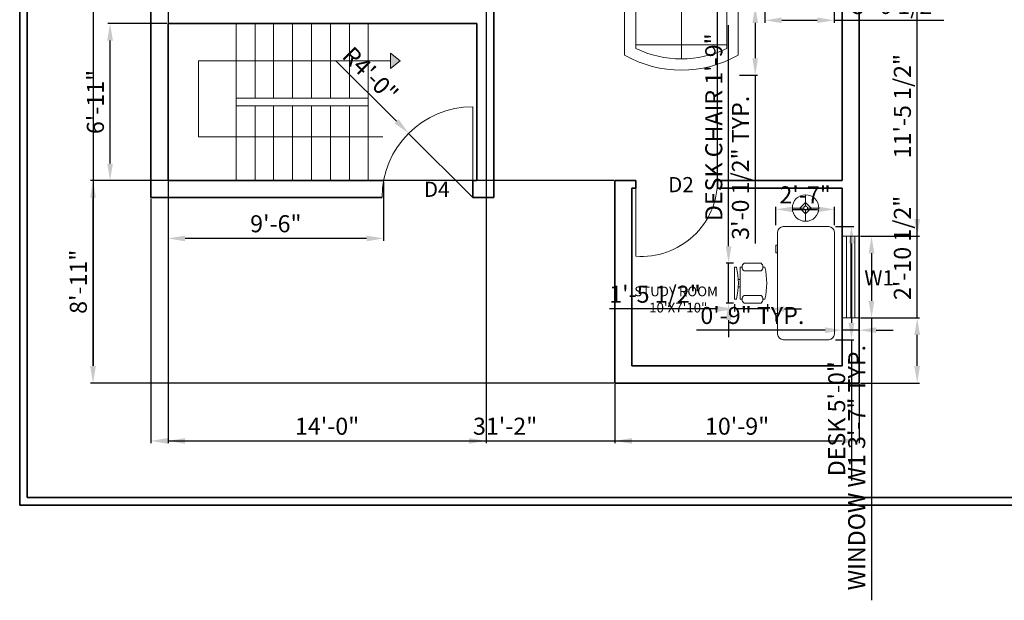
# Model space of a CAD drawing. Units: inches. Extents: x 2396 to 4051, y 1419 to 2191.
# Tile 1 of 7: x 2461 to 2981, y 1419 to 1726. Entities that reach past the tile are written whole.
import ezdxf

# ---------------------------------------------------------------- set-up
doc = ezdxf.new("R2010")
doc.units = ezdxf.units.IN
for name, color, linetype, lineweight in [('A-ANNO-SYMB', 3, 'Continuous', 13), ('A-ANNO-TTLB', 7, 'Continuous', 35), ('A-AREA-IDEN', 6, 'Continuous', 18), ('A-DOOR', 4, 'Continuous', 18), ('A-FLOR-STRS', 7, 'Continuous', 18), ('A-FURN', 8, 'Continuous', 18), ('A-WALL', 7, 'Continuous', 35), ('S-ANNO-DIMS', 2, 'Continuous', 18)]:
    doc.layers.add(name, color=color, linetype=linetype, lineweight=lineweight)
doc.layers.add('A-ANNO-TEXT', color=114, linetype='Continuous', lineweight=18, true_color=0x139b48)
doc.layers.add('A-GLAZ', color=52, linetype='Continuous', lineweight=18, true_color=0xc8c92d)
doc.styles.get("Standard").update_dxf_attribs({"font": 'arial.ttf'})
doc.dimstyles.new('ISO-25', dxfattribs={"dimtxt": 9, "dimasz": 9, "dimexe": 1.25, "dimexo": 0.625, "dimgap": 2, "dimtad": 1, "dimdec": 1, "dimlunit": 4, "dimtxsty": 'Standard', "dimcen": 2.5, "dimadec": 0, "dimazin": 0, "dimtfac": 1, "dimtdec": 1, "dimtmove": 0, "dimatfit": 3, "dimfxl": 1, "dimarcsym": 0})

# ---------------------------------------------------------------- blocks, each defined once
blk = doc.blocks.new('Sofa - Roundback Loveseat 5 ft.')
for p, q in [((0, -32.44198), (0, -5.99998)), ((-24, -33.99998), (-24, -11.46958)), ((-23.9998, -13.38178), (23.99986, -13.38178)), ((24.00004, -33.99998), (24.00004, -11.46958)), ((-24, -32.44198), (24.00004, -32.44198))]:
    blk.add_line(p, q)
for points in [[(-24, -33.99998), (-30, -33.99998), (-30, -7.99998)], [(30.00004, -7.99998), (30.00004, -33.99998), (24.00004, -33.99998)]]:
    blk.add_lwpolyline(points)
for centre, radius, start, end in [((0, -60.24998), 60.24998, 60.13715, 119.8628), ((0, -61.38438), 55.38444, 64.32083, 115.6792)]:
    blk.add_arc(centre, radius, start, end)
blk = doc.blocks.new('Desk - 30 x 60 in.')
for p, q in [((-26.999995, 0), (26.999995, 0)), ((-29.999995, -27), (-29.999995, -3)), ((29.999995, -3), (29.999995, -27)), ((26.999995, -30), (-26.999995, -30)), ((-20.000005, -30), (-20.000005, -31)), ((-20.000005, -31), (-16.000005, -31)), ((-16.000005, -31), (-16.000005, -30)), ((15.999995, -31), (15.999995, -30)), ((19.999995, -31), (15.999995, -31)), ((19.999995, -30), (19.999995, -31))]:
    blk.add_line(p, q)
for centre, start, end in [((-26.499995, -3.5), 98.1301, 171.8699), ((26.499995, -3.5), 8.130102, 81.8699), ((-26.499995, -26.5), 188.1301, 261.8699), ((26.499995, -26.5), 278.1301, 351.8699)]:
    blk.add_arc(centre, 3.535534, start, end)
blk = doc.blocks.new('Lamp - Table')
for p, q in [((0, 7), (0, 1)), ((-1, 0), (-7, 0)), ((0, 3), (-3, 0)), ((-3, 0), (0, -3)), ((3, 0), (0, 3)), ((0, -3), (3, 0)), ((1, 0), (7, 0)), ((0, -1), (0, -7))]:
    blk.add_line(p, q)
for radius in [7, 1]:
    blk.add_circle((0, 0), radius)
blk = doc.blocks.new('Chair - Desk')
for p, q in [((-8.5, 0), (-8.5, -1)), ((-8.5, 0), (8.5, 0)), ((8.5, 0), (8.5, -1)), ((-10.5, -5), (-10.5, -14)), ((-8.5, -3), (-8.5, -4)), ((-8.5, -3), (8.5, -3)), ((-6.5, -14), (-6.5, -5)), ((-2, -3), (-2, -1.9355)), ((2, -1.9576), (2, -3)), ((6.5, -5), (6.5, -14)), ((8.5, -3), (8.5, -4)), ((10.5, -14), (10.5, -5)), ((-8.5, -15), (-8.5, -16)), ((8.5, -15), (8.5, -16))]:
    blk.add_line(p, q)
for centre, radius, start, end in [((-8.5, -6.5), 2.5, 36.8699, 143.1301), ((0, 34.625), 36.625, 256.5803, 283.4197), ((8.5, -6.5), 2.5, 36.8699, 143.1301), ((-8.5, -12.5), 2.5, 216.8699, 323.1301), ((8.5, -12.5), 2.5, 216.8699, 323.1301), ((0, 19.625), 36.625, 256.5803, 283.4197)]:
    blk.add_arc(centre, radius, start, end)
blk = doc.blocks.new('WIN-W1-43P2IN')
for p, q in [((9, 43.2), (0, 43.2)), ((2.25, 0), (2.25, 43.2)), ((4.5, 0), (4.5, 43.2)), ((6.75, 0), (6.75, 43.2)), ((9, 0), (0, 0))]:
    blk.add_line(p, q)
blk = doc.blocks.new('DOOR-D2-40IN')
blk.add_line((0, 40.11), (0, 0.11))
blk.add_arc((3.08, 40.11), 40.12, 265.5948, 0)
blk = doc.blocks.new('*D45')
at = {"layer": 'Defpoints', "color": 0, "transparency": 16777216}
for p in [(2840.06, 1733.59), (2840.06, 1696.93), (2849.06, 1696.93)]:
    blk.add_point(p, dxfattribs=at)
at = {"layer": 'S-ANNO-DIMS', "color": 0, "lineweight": -2, "transparency": 16777216}
for p, q in [((2840.69, 1733.59), (2850.31, 1733.59)), ((2849.06, 1724.59), (2849.06, 1705.93)), ((2840.69, 1696.93), (2850.31, 1696.93)), ((2849.06, 1696.93), (2849.06, 1608.1))]:
    blk.add_line(p, q, dxfattribs=at)
at = {"layer": 'S-ANNO-DIMS', "color": 0, "transparency": 16777216}
for points in [[(2847.56, 1724.59), (2850.56, 1724.59), (2849.06, 1733.59)], [(2847.56, 1705.93), (2850.56, 1705.93), (2849.06, 1696.93)]]:
    blk.add_solid(points, dxfattribs=at)
at = {"layer": 'S-ANNO-DIMS', "color": 0, "transparency": 16777216, "insert": (2842.41, 1648.02), "char_height": 9, "attachment_point": 5, "rotation": 90}
blk.add_mtext('3\'-0 1/2" TYP.', dxfattribs=at)
blk = doc.blocks.new('*D54')
at = {"layer": 'Defpoints', "color": 0, "transparency": 16777216}
for p in [(2903.98, 1611.9), (2903.98, 1568.7), (2910.46, 1568.7)]:
    blk.add_point(p, dxfattribs=at)
at = {"layer": 'S-ANNO-DIMS', "color": 0, "lineweight": -2, "transparency": 16777216}
for p, q in [((2904.61, 1611.9), (2911.71, 1611.9)), ((2910.46, 1602.9), (2910.46, 1577.7)), ((2904.61, 1568.7), (2911.71, 1568.7)), ((2910.46, 1568.7), (2910.46, 1419.46))]:
    blk.add_line(p, q, dxfattribs=at)
at = {"layer": 'S-ANNO-DIMS', "color": 0, "transparency": 16777216}
for points in [[(2908.96, 1602.9), (2911.96, 1602.9), (2910.46, 1611.9)], [(2908.96, 1577.7), (2911.96, 1577.7), (2910.46, 1568.7)]]:
    blk.add_solid(points, dxfattribs=at)
at = {"layer": 'S-ANNO-DIMS', "color": 0, "transparency": 16777216, "insert": (2903.8, 1489.58), "char_height": 9, "attachment_point": 5, "rotation": 90}
blk.add_mtext('WINDOW W1 3\'-7" TYP.', dxfattribs=at)
blk = doc.blocks.new('*D55')
at = {"layer": 'Defpoints', "color": 0, "transparency": 16777216}
for p in [(2894.98, 1568.7), (2903.98, 1568.7), (2894.98, 1562.22)]:
    blk.add_point(p, dxfattribs=at)
at = {"layer": 'S-ANNO-DIMS', "color": 0, "lineweight": -2, "transparency": 16777216}
for p, q in [((2894.98, 1568.08), (2894.98, 1560.97)), ((2903.98, 1568.08), (2903.98, 1560.97)), ((2885.98, 1562.22), (2818.12, 1562.22)), ((2903.98, 1562.22), (2894.98, 1562.22)), ((2912.98, 1562.22), (2921.98, 1562.22))]:
    blk.add_line(p, q, dxfattribs=at)
at = {"layer": 'S-ANNO-DIMS', "color": 0, "transparency": 16777216}
for points in [[(2885.98, 1563.72), (2885.98, 1560.72), (2894.98, 1562.22)], [(2912.98, 1563.72), (2912.98, 1560.72), (2903.98, 1562.22)]]:
    blk.add_solid(points, dxfattribs=at)
at = {"layer": 'S-ANNO-DIMS', "color": 0, "transparency": 16777216, "insert": (2847.55, 1568.82), "char_height": 9, "attachment_point": 5}
blk.add_mtext('0\'-9" TYP.', dxfattribs=at)
blk = doc.blocks.new('*D63')
at = {"layer": 'Defpoints', "color": 0, "transparency": 16777216}
for p in [(2854.1, 1738.57), (2890.77, 1738.57), (2890.77, 1725.97)]:
    blk.add_point(p, dxfattribs=at)
at = {"layer": 'S-ANNO-DIMS', "color": 0, "lineweight": -2, "transparency": 16777216}
for p, q in [((2854.1, 1737.94), (2854.1, 1724.72)), ((2890.77, 1737.94), (2890.77, 1724.72)), ((2863.1, 1725.97), (2881.77, 1725.97)), ((2890.77, 1725.97), (2948.66, 1725.97))]:
    blk.add_line(p, q, dxfattribs=at)
at = {"layer": 'S-ANNO-DIMS', "color": 0, "transparency": 16777216}
for points in [[(2863.1, 1727.47), (2863.1, 1724.47), (2854.1, 1725.97)], [(2881.77, 1727.47), (2881.77, 1724.47), (2890.77, 1725.97)]]:
    blk.add_solid(points, dxfattribs=at)
at = {"layer": 'S-ANNO-DIMS', "color": 0, "transparency": 16777216, "insert": (2924.21, 1732.63), "char_height": 9, "attachment_point": 5}
blk.add_mtext('3\'-0 1/2"', dxfattribs=at)
blk = doc.blocks.new('*D64')
at = {"layer": 'Defpoints', "color": 0, "transparency": 16777216}
for p in [(2890.89, 1617.07), (2890.89, 1557.07), (2899.89, 1557.07)]:
    blk.add_point(p, dxfattribs=at)
at = {"layer": 'S-ANNO-DIMS', "color": 0, "lineweight": -2, "transparency": 16777216}
for p, q in [((2891.51, 1617.07), (2901.14, 1617.07)), ((2899.89, 1608.07), (2899.89, 1566.07)), ((2891.51, 1557.07), (2901.14, 1557.07)), ((2899.89, 1557.07), (2899.89, 1482.86))]:
    blk.add_line(p, q, dxfattribs=at)
at = {"layer": 'S-ANNO-DIMS', "color": 0, "transparency": 16777216}
for points in [[(2898.39, 1608.07), (2901.39, 1608.07), (2899.89, 1617.07)], [(2898.39, 1566.07), (2901.39, 1566.07), (2899.89, 1557.07)]]:
    blk.add_solid(points, dxfattribs=at)
at = {"layer": 'S-ANNO-DIMS', "color": 0, "transparency": 16777216, "insert": (2893.23, 1515.46), "char_height": 9, "attachment_point": 5, "rotation": 90}
blk.add_mtext('DESK 5\'-0"', dxfattribs=at)
blk = doc.blocks.new('*D65')
at = {"layer": 'Defpoints', "color": 0, "transparency": 16777216}
for p in [(2890.89, 1626.07), (2859.89, 1617.07), (2890.89, 1617.07)]:
    blk.add_point(p, dxfattribs=at)
at = {"layer": 'S-ANNO-DIMS', "color": 0, "lineweight": -2, "transparency": 16777216}
for p, q in [((2859.89, 1617.69), (2859.89, 1627.32)), ((2868.89, 1626.07), (2881.89, 1626.07)), ((2890.89, 1617.69), (2890.89, 1627.32))]:
    blk.add_line(p, q, dxfattribs=at)
at = {"layer": 'S-ANNO-DIMS', "color": 0, "transparency": 16777216}
for points in [[(2868.89, 1627.57), (2868.89, 1624.57), (2859.89, 1626.07)], [(2881.89, 1627.57), (2881.89, 1624.57), (2890.89, 1626.07)]]:
    blk.add_solid(points, dxfattribs=at)
at = {"layer": 'S-ANNO-DIMS', "color": 0, "transparency": 16777216, "insert": (2875.39, 1632.58), "char_height": 9, "attachment_point": 5}
blk.add_mtext('2\'-7"', dxfattribs=at)
blk = doc.blocks.new('*D70')
at = {"layer": 'Defpoints', "color": 0, "transparency": 16777216}
for p in [(2834.99, 1597.57), (2838.14, 1597.57), (2838.14, 1576.57)]:
    blk.add_point(p, dxfattribs=at)
at = {"layer": 'S-ANNO-DIMS', "color": 0, "lineweight": -2, "transparency": 16777216}
for p, q in [((2834.99, 1606.57), (2834.99, 1723.39)), ((2837.52, 1597.57), (2833.74, 1597.57)), ((2834.99, 1576.57), (2834.99, 1597.57)), ((2837.52, 1576.57), (2833.74, 1576.57)), ((2834.99, 1567.57), (2834.99, 1558.57))]:
    blk.add_line(p, q, dxfattribs=at)
at = {"layer": 'S-ANNO-DIMS', "color": 0, "transparency": 16777216}
for points in [[(2833.49, 1606.57), (2836.49, 1606.57), (2834.99, 1597.57)], [(2833.49, 1567.57), (2836.49, 1567.57), (2834.99, 1576.57)]]:
    blk.add_solid(points, dxfattribs=at)
at = {"layer": 'S-ANNO-DIMS', "color": 0, "transparency": 16777216, "insert": (2828.34, 1669.48), "char_height": 9, "attachment_point": 5, "rotation": 90}
blk.add_mtext('DESK CHAIR 1\'-9"', dxfattribs=at)
blk = doc.blocks.new('*D71')
at = {"layer": 'Defpoints', "color": 0, "transparency": 16777216}
for p in [(2838.14, 1576.57), (2855.48, 1576.57), (2838.14, 1573.42)]:
    blk.add_point(p, dxfattribs=at)
at = {"layer": 'S-ANNO-DIMS', "color": 0, "lineweight": -2, "transparency": 16777216}
for p, q in [((2838.14, 1575.94), (2838.14, 1572.17)), ((2855.48, 1575.94), (2855.48, 1572.17)), ((2829.14, 1573.42), (2772.09, 1573.42)), ((2855.48, 1573.42), (2838.14, 1573.42)), ((2864.48, 1573.42), (2873.48, 1573.42))]:
    blk.add_line(p, q, dxfattribs=at)
at = {"layer": 'S-ANNO-DIMS', "color": 0, "transparency": 16777216}
for points in [[(2829.14, 1574.92), (2829.14, 1571.92), (2838.14, 1573.42)], [(2864.48, 1574.92), (2864.48, 1571.92), (2855.48, 1573.42)]]:
    blk.add_solid(points, dxfattribs=at)
at = {"layer": 'S-ANNO-DIMS', "color": 0, "transparency": 16777216, "insert": (2796.12, 1580.07), "char_height": 9, "attachment_point": 5}
blk.add_mtext('1\'-5 1/2"', dxfattribs=at)
blk = doc.blocks.new('*D76')
at = {"layer": 'Defpoints', "color": 0, "transparency": 16777216}
for p in [(2529.98, 1632.3), (2903.98, 1534.3), (2903.98, 1503.7)]:
    blk.add_point(p, dxfattribs=at)
at = {"layer": 'S-ANNO-DIMS', "color": 0, "lineweight": -2, "transparency": 16777216}
for p, q in [((2529.98, 1631.68), (2529.98, 1502.45)), ((2903.98, 1533.68), (2903.98, 1502.45)), ((2538.98, 1503.7), (2894.98, 1503.7))]:
    blk.add_line(p, q, dxfattribs=at)
at = {"layer": 'S-ANNO-DIMS', "color": 0, "transparency": 16777216}
for points in [[(2538.98, 1505.2), (2538.98, 1502.2), (2529.98, 1503.7)], [(2894.98, 1505.2), (2894.98, 1502.2), (2903.98, 1503.7)]]:
    blk.add_solid(points, dxfattribs=at)
at = {"layer": 'S-ANNO-DIMS', "color": 0, "transparency": 16777216, "insert": (2716.98, 1510.3), "char_height": 9, "attachment_point": 5}
blk.add_mtext('31\'-2"', dxfattribs=at)
blk = doc.blocks.new('*D77')
at = {"layer": 'Defpoints', "color": 0, "transparency": 16777216}
for p in [(2529.98, 2074.3), (2499.38, 1534.3), (2774.98, 1534.3)]:
    blk.add_point(p, dxfattribs=at)
at = {"layer": 'S-ANNO-DIMS', "color": 0, "lineweight": -2, "transparency": 16777216}
for p, q in [((2529.36, 2074.3), (2498.13, 2074.3)), ((2499.38, 2065.3), (2499.38, 1543.3)), ((2774.36, 1534.3), (2498.13, 1534.3))]:
    blk.add_line(p, q, dxfattribs=at)
at = {"layer": 'S-ANNO-DIMS', "color": 0, "transparency": 16777216}
for points in [[(2497.88, 2065.3), (2500.88, 2065.3), (2499.38, 2074.3)], [(2497.88, 1543.3), (2500.88, 1543.3), (2499.38, 1534.3)]]:
    blk.add_solid(points, dxfattribs=at)
at = {"layer": 'S-ANNO-DIMS', "color": 0, "transparency": 16777216, "insert": (2492.79, 1804.3), "char_height": 9, "attachment_point": 5, "rotation": 90}
blk.add_mtext('45\'-0"', dxfattribs=at)
blk = doc.blocks.new('*D78')
at = {"layer": 'Defpoints', "color": 0, "transparency": 16777216}
for p in [(2538.98, 1733.3), (2706.98, 1733.3), (2706.98, 1503.7)]:
    blk.add_point(p, dxfattribs=at)
at = {"layer": 'S-ANNO-DIMS', "color": 0, "lineweight": -2, "transparency": 16777216}
for p, q in [((2538.98, 1732.68), (2538.98, 1502.45)), ((2706.98, 1732.68), (2706.98, 1502.45)), ((2547.98, 1503.7), (2697.98, 1503.7))]:
    blk.add_line(p, q, dxfattribs=at)
at = {"layer": 'S-ANNO-DIMS', "color": 0, "transparency": 16777216}
for points in [[(2547.98, 1505.2), (2547.98, 1502.2), (2538.98, 1503.7)], [(2697.98, 1505.2), (2697.98, 1502.2), (2706.98, 1503.7)]]:
    blk.add_solid(points, dxfattribs=at)
at = {"layer": 'S-ANNO-DIMS', "color": 0, "transparency": 16777216, "insert": (2622.98, 1510.3), "char_height": 9, "attachment_point": 5}
blk.add_mtext('14\'-0"', dxfattribs=at)
blk = doc.blocks.new('*D79')
at = {"layer": 'Defpoints', "color": 0, "transparency": 16777216}
for p in [(2774.98, 1534.3), (2903.98, 1534.3), (2903.98, 1503.7)]:
    blk.add_point(p, dxfattribs=at)
at = {"layer": 'S-ANNO-DIMS', "color": 0, "lineweight": -2, "transparency": 16777216}
for p, q in [((2774.98, 1533.68), (2774.98, 1502.45)), ((2903.98, 1533.68), (2903.98, 1502.45)), ((2783.98, 1503.7), (2894.98, 1503.7))]:
    blk.add_line(p, q, dxfattribs=at)
at = {"layer": 'S-ANNO-DIMS', "color": 0, "transparency": 16777216}
for points in [[(2783.98, 1505.2), (2783.98, 1502.2), (2774.98, 1503.7)], [(2894.98, 1505.2), (2894.98, 1502.2), (2903.98, 1503.7)]]:
    blk.add_solid(points, dxfattribs=at)
at = {"layer": 'S-ANNO-DIMS', "color": 0, "transparency": 16777216, "insert": (2839.48, 1510.3), "char_height": 9, "attachment_point": 5}
blk.add_mtext('10\'-9"', dxfattribs=at)
blk = doc.blocks.new('*D80')
at = {"layer": 'Defpoints', "color": 0, "transparency": 16777216}
for p in [(2499.38, 1641.3), (2774.98, 1641.3), (2774.98, 1534.3)]:
    blk.add_point(p, dxfattribs=at)
at = {"layer": 'S-ANNO-DIMS', "color": 0, "lineweight": -2, "transparency": 16777216}
for p, q in [((2774.36, 1641.3), (2498.13, 1641.3)), ((2499.38, 1543.3), (2499.38, 1632.3)), ((2774.36, 1534.3), (2498.13, 1534.3))]:
    blk.add_line(p, q, dxfattribs=at)
at = {"layer": 'S-ANNO-DIMS', "color": 0, "transparency": 16777216}
for points in [[(2497.88, 1632.3), (2500.88, 1632.3), (2499.38, 1641.3)], [(2497.88, 1543.3), (2500.88, 1543.3), (2499.38, 1534.3)]]:
    blk.add_solid(points, dxfattribs=at)
at = {"layer": 'S-ANNO-DIMS', "color": 0, "transparency": 16777216, "insert": (2492.79, 1587.8), "char_height": 9, "attachment_point": 5, "rotation": 90}
blk.add_mtext('8\'-11"', dxfattribs=at)
blk = doc.blocks.new('*D82')
at = {"layer": 'Defpoints', "color": 0, "transparency": 16777216}
for p in [(2903.98, 1749.3), (2934.58, 1749.3), (2903.98, 1611.9)]:
    blk.add_point(p, dxfattribs=at)
at = {"layer": 'S-ANNO-DIMS', "color": 0, "lineweight": -2, "transparency": 16777216}
for p, q in [((2904.61, 1749.3), (2935.83, 1749.3)), ((2934.58, 1620.9), (2934.58, 1740.3)), ((2904.61, 1611.9), (2935.83, 1611.9))]:
    blk.add_line(p, q, dxfattribs=at)
at = {"layer": 'S-ANNO-DIMS', "color": 0, "transparency": 16777216}
for points in [[(2933.08, 1740.3), (2936.08, 1740.3), (2934.58, 1749.3)], [(2933.08, 1620.9), (2936.08, 1620.9), (2934.58, 1611.9)]]:
    blk.add_solid(points, dxfattribs=at)
at = {"layer": 'S-ANNO-DIMS', "color": 0, "transparency": 16777216, "insert": (2927.93, 1680.6), "char_height": 9, "attachment_point": 5, "rotation": 90}
blk.add_mtext('11\'-5 1/2"', dxfattribs=at)
blk = doc.blocks.new('*D88')
at = {"layer": 'Defpoints', "color": 0, "transparency": 16777216}
for p in [(2903.98, 1568.7), (2934.58, 1568.7), (2903.98, 1534.3)]:
    blk.add_point(p, dxfattribs=at)
at = {"layer": 'S-ANNO-DIMS', "color": 0, "lineweight": -2, "transparency": 16777216}
for p, q in [((2934.58, 1568.7), (2934.58, 1633.74)), ((2904.61, 1568.7), (2935.83, 1568.7)), ((2934.58, 1543.3), (2934.58, 1559.7)), ((2904.61, 1534.3), (2935.83, 1534.3))]:
    blk.add_line(p, q, dxfattribs=at)
at = {"layer": 'S-ANNO-DIMS', "color": 0, "transparency": 16777216}
for points in [[(2933.08, 1559.7), (2936.08, 1559.7), (2934.58, 1568.7)], [(2933.08, 1543.3), (2936.08, 1543.3), (2934.58, 1534.3)]]:
    blk.add_solid(points, dxfattribs=at)
at = {"layer": 'S-ANNO-DIMS', "color": 0, "transparency": 16777216, "insert": (2927.93, 1605.72), "char_height": 9, "attachment_point": 5, "rotation": 90}
blk.add_mtext('2\'-10 1/2"', dxfattribs=at)
blk = doc.blocks.new('*D90')
at = {"layer": 'Defpoints', "color": 0, "transparency": 16777216}
for p in [(2508.38, 1724.3), (2538.98, 1724.3), (2538.98, 1641.3)]:
    blk.add_point(p, dxfattribs=at)
at = {"layer": 'S-ANNO-DIMS', "color": 0, "lineweight": -2, "transparency": 16777216}
for p, q in [((2538.36, 1724.3), (2507.13, 1724.3)), ((2508.38, 1650.3), (2508.38, 1715.3)), ((2538.36, 1641.3), (2507.13, 1641.3))]:
    blk.add_line(p, q, dxfattribs=at)
at = {"layer": 'S-ANNO-DIMS', "color": 0, "transparency": 16777216}
for points in [[(2506.88, 1715.3), (2509.88, 1715.3), (2508.38, 1724.3)], [(2506.88, 1650.3), (2509.88, 1650.3), (2508.38, 1641.3)]]:
    blk.add_solid(points, dxfattribs=at)
at = {"layer": 'S-ANNO-DIMS', "color": 0, "transparency": 16777216, "insert": (2501.79, 1682.8), "char_height": 9, "attachment_point": 5, "rotation": 90}
blk.add_mtext('6\'-11"', dxfattribs=at)
blk = doc.blocks.new('*D93')
at = {"layer": 'Defpoints', "color": 0, "transparency": 16777216}
for p in [(2538.98, 1641.3), (2652.84, 1641.3), (2538.98, 1610.7)]:
    blk.add_point(p, dxfattribs=at)
at = {"layer": 'S-ANNO-DIMS', "color": 0, "lineweight": -2, "transparency": 16777216}
for p, q in [((2538.98, 1640.68), (2538.98, 1609.45)), ((2652.84, 1640.68), (2652.84, 1609.45)), ((2643.84, 1610.7), (2547.98, 1610.7))]:
    blk.add_line(p, q, dxfattribs=at)
at = {"layer": 'S-ANNO-DIMS', "color": 0, "transparency": 16777216}
for points in [[(2547.98, 1612.2), (2547.98, 1609.2), (2538.98, 1610.7)], [(2643.84, 1612.2), (2643.84, 1609.2), (2652.84, 1610.7)]]:
    blk.add_solid(points, dxfattribs=at)
at = {"layer": 'S-ANNO-DIMS', "color": 0, "transparency": 16777216, "insert": (2595.91, 1617.3), "char_height": 9, "attachment_point": 5}
blk.add_mtext('9\'-6"', dxfattribs=at)
blk = doc.blocks.new('*D96')
at = {"layer": 'Defpoints', "color": 0, "transparency": 16777216}
for p in [(2894.98, 2154.77), (2829.18, 1641.3), (2894.98, 1641.3)]:
    blk.add_point(p, dxfattribs=at)
at = {"layer": 'S-ANNO-DIMS', "color": 0, "lineweight": -2, "transparency": 16777216}
for p, q in [((2829.18, 1641.93), (2829.18, 2156.02)), ((2838.18, 2154.77), (2885.98, 2154.77)), ((2894.98, 1641.93), (2894.98, 2156.02))]:
    blk.add_line(p, q, dxfattribs=at)
at = {"layer": 'S-ANNO-DIMS', "color": 0, "transparency": 16777216}
for points in [[(2838.18, 2156.27), (2838.18, 2153.27), (2829.18, 2154.77)], [(2885.98, 2156.27), (2885.98, 2153.27), (2894.98, 2154.77)]]:
    blk.add_solid(points, dxfattribs=at)
at = {"layer": 'S-ANNO-DIMS', "color": 0, "transparency": 16777216, "insert": (2862.08, 2161.37), "char_height": 9, "attachment_point": 5}
blk.add_mtext('5\'-6"', dxfattribs=at)
blk = doc.blocks.new('*D112')
at = {"layer": 'Defpoints', "color": 0, "transparency": 16777216}
for p in [(2666.04, 1666.24), (2699.98, 1632.3)]:
    blk.add_point(p, dxfattribs=at)
at = {"layer": 'S-ANNO-DIMS', "color": 0, "lineweight": -2, "transparency": 16777216}
for p, q in [((2627.48, 1704.81), (2659.68, 1672.61)), ((2699.98, 1632.3), (2666.04, 1666.24))]:
    blk.add_line(p, q, dxfattribs=at)
at = {"layer": 'S-ANNO-DIMS', "color": 0, "transparency": 16777216}
blk.add_solid([(2660.74, 1673.67), (2658.62, 1671.55), (2666.04, 1666.24)], dxfattribs=at)
at = {"layer": 'S-ANNO-DIMS', "color": 0, "transparency": 16777216, "insert": (2645.06, 1696.55), "char_height": 9, "attachment_point": 5, "rotation": 314.9996}
blk.add_mtext('R4\'-0"', dxfattribs=at)

msp = doc.modelspace()

# ---------------------------------------------------------------- hatches: boundary and pattern name
at = {"layer": 'A-ANNO-SYMB'}
h = msp.add_hatch(color=256, dxfattribs=at)
h.dxf.hatch_style = 1
h.paths.add_polyline_path([(2656.48, 1708.55), (2656.48, 1704.55), (2656.48, 1700.55), (2661.48, 1704.55)])

# ---------------------------------------------------------------- linework, layer by layer
for p, q in [((2656.48, 1704.55), (2656.48, 1708.55)), ((2656.48, 1708.55), (2661.48, 1704.55)), ((2555.1, 1664.38), (2555.1, 1704.55)), ((2555.1, 1704.55), (2656.48, 1704.55)), ((2656.48, 1704.55), (2656.48, 1700.55)), ((2661.48, 1704.55), (2656.48, 1700.55)), ((2652.49, 1664.38), (2555.1, 1664.38))]:
    msp.add_line(p, q, dxfattribs=at)
at = {"layer": 'A-ANNO-TTLB'}
for points in [[(2460.66, 2191.26), (4051.21, 2191.26), (4051.21, 1469.82), (2460.66, 1469.82)], [(2464.66, 2187.26), (4047.21, 2187.26), (4047.21, 1473.82), (2464.66, 1473.82)]]:
    msp.add_lwpolyline(points, close=True, dxfattribs=at)
at = {"layer": 'A-DOOR'}
msp.add_line((2699.98, 1680.3), (2699.98, 1632.3), dxfattribs=at)
msp.add_arc((2699.98, 1632.3), 48, 90, 180, dxfattribs=at)
at = {"layer": 'A-FLOR-STRS'}
for p, q in [((2574.98, 1641.3), (2574.98, 1724.3)), ((2584.98, 1684.8), (2584.98, 1724.3)), ((2594.74, 1684.8), (2594.74, 1724.3)), ((2604.74, 1684.8), (2604.74, 1724.3)), ((2614.74, 1684.8), (2614.74, 1724.3)), ((2624.74, 1684.8), (2624.74, 1724.3)), ((2634.74, 1684.8), (2634.74, 1724.3)), ((2644.74, 1641.3), (2644.74, 1724.3)), ((2574.98, 1684.8), (2644.74, 1684.8)), ((2574.98, 1680.8), (2644.74, 1680.8)), ((2584.98, 1641.3), (2584.98, 1680.8)), ((2594.74, 1641.3), (2594.74, 1680.8)), ((2604.74, 1641.3), (2604.74, 1680.8)), ((2614.74, 1641.3), (2614.74, 1680.8)), ((2624.74, 1641.3), (2624.74, 1680.8)), ((2634.74, 1641.3), (2634.74, 1680.8))]:
    msp.add_line(p, q, dxfattribs=at)
at = {"layer": 'A-WALL'}
for p, q in [((2529.98, 1632.3), (2529.98, 2074.3)), ((2903.98, 2074.3), (2903.98, 1534.3)), ((2894.98, 1917.3), (2894.98, 1641.3)), ((2710.98, 1857.3), (2710.98, 1632.3)), ((2538.98, 1641.3), (2538.98, 1724.3)), ((2701.98, 1724.3), (2538.98, 1724.3)), ((2701.98, 1724.3), (2701.98, 1641.3)), ((2652.84, 1641.3), (2538.98, 1641.3)), ((2701.98, 1641.3), (2699.98, 1641.3)), ((2699.98, 1641.3), (2699.98, 1632.3)), ((2774.98, 1641.3), (2774.98, 1534.3)), ((2785.98, 1641.3), (2774.98, 1641.3)), ((2785.98, 1641.3), (2785.98, 1637.3)), ((2894.98, 1641.3), (2829.18, 1641.3)), ((2829.18, 1641.3), (2829.18, 1637.3)), ((2783.98, 1637.3), (2783.98, 1543.3)), ((2785.98, 1637.3), (2783.98, 1637.3)), ((2894.98, 1637.3), (2829.18, 1637.3)), ((2894.98, 1637.3), (2894.98, 1543.3)), ((2651.98, 1632.3), (2529.98, 1632.3)), ((2710.98, 1632.3), (2699.98, 1632.3)), ((2894.98, 1543.3), (2783.98, 1543.3)), ((2903.98, 1534.3), (2774.98, 1534.3))]:
    msp.add_line(p, q, dxfattribs=at)

# ---------------------------------------------------------------- block references
at = {"layer": 'A-DOOR'}
msp.add_blockref('DOOR-D2-40IN', (2785.98, 1601.19), dxfattribs=at)
at = {"layer": 'A-FURN', "xscale": -1, "rotation": 180}
msp.add_blockref('Sofa - Roundback Loveseat 5 ft.', (2810.06, 1699.59), dxfattribs=at)
at = {"layer": 'A-FURN'}
msp.add_blockref('Lamp - Table', (2875.67, 1626.77), dxfattribs=at)
for name, p, rotation in [('Desk - 30 x 60 in.', (2890.89, 1587.07), 270), ('Chair - Desk', (2838.14, 1587.07), 90)]:
    msp.add_blockref(name, p, dxfattribs=dict(at, rotation=rotation))
at = {"layer": 'A-GLAZ', "rotation": 180}
msp.add_blockref('WIN-W1-43P2IN', (2903.98, 1611.9), dxfattribs=at)

# ---------------------------------------------------------------- texts
at = {"layer": 'A-ANNO-TEXT', "char_height": 8, "attachment_point": 1}
for s, insert in [('{D2}', (2803.06, 1643.14)), ('{D4}', (2674.08, 1640.68)), ('W1', (2906.67, 1593.86))]:
    msp.add_mtext_dynamic_manual_height_columns(s, width=139.3028, gutter_width=12.5, heights=[0], dxfattribs=dict(at, insert=insert))
at = {"layer": 'A-AREA-IDEN', "insert": (2780.49, 1585.29), "char_height": 5.142, "attachment_point": 1}
msp.add_mtext_dynamic_manual_height_columns('   STUDY ROOM\\P        10\'X7\'10"', width=89.5376, gutter_width=8.03, heights=[0], dxfattribs=at)

# ---------------------------------------------------------------- dimensions: what is measured, and where the dimension line sits
at = {"layer": 'S-ANNO-DIMS'}
for base, p1, p2, picture, middle in [((2894.98, 2154.77), (2829.18, 1641.3), (2894.98, 1641.3), '*D96', (2862.08, 2161.37)), ((2890.77, 1725.97), (2854.1, 1738.57), (2890.77, 1738.57), '*D63', (2924.21, 1732.63)), ((2706.98, 1503.7), (2538.98, 1733.3), (2706.98, 1733.3), '*D78', (2622.98, 1510.3)), ((2890.89, 1626.07), (2859.89, 1617.07), (2890.89, 1617.07), '*D65', (2875.39, 1632.58)), ((2903.98, 1503.7), (2529.98, 1632.3), (2903.98, 1534.3), '*D76', (2716.98, 1510.3)), ((2903.98, 1503.7), (2774.98, 1534.3), (2903.98, 1534.3), '*D79', (2839.48, 1510.3))]:
    dim = msp.add_linear_dim(base=base, p1=p1, p2=p2, dimstyle='ISO-25', override={"dimdec": 1, "dimlfac": 1, "dimrnd": 0, "dimzin": 1, "dimdsep": 46, "dimlunit": 4, "dimfrac": 2}, dxfattribs=at)
    dim.commit()
    dim.dimension.update_dxf_attribs({"geometry": picture, "text_midpoint": middle})
for base, p1, p2, angle, picture, middle in [((2499.38, 1534.3), (2529.98, 2074.3), (2774.98, 1534.3), 90, '*D77', (2492.79, 1804.3)), ((2934.58, 1749.3), (2903.98, 1611.9), (2903.98, 1749.3), 90, '*D82', (2927.93, 1680.6)), ((2508.38, 1724.3), (2538.98, 1641.3), (2538.98, 1724.3), 90, '*D90', (2501.79, 1682.8)), ((2499.38, 1641.3), (2774.98, 1534.3), (2774.98, 1641.3), 90, '*D80', (2492.79, 1587.8)), ((2538.98, 1610.7), (2652.84, 1641.3), (2538.98, 1641.3), 180, '*D93', (2595.91, 1617.3)), ((2934.58, 1568.7), (2903.98, 1534.3), (2903.98, 1568.7), 90, '*D88', (2927.93, 1605.72)), ((2838.14, 1573.42), (2855.48, 1576.57), (2838.14, 1576.57), 180, '*D71', (2796.12, 1580.07))]:
    dim = msp.add_linear_dim(base=base, p1=p1, p2=p2, angle=angle, dimstyle='ISO-25', override={"dimdec": 1, "dimlfac": 1, "dimrnd": 0, "dimzin": 1, "dimdsep": 46, "dimlunit": 4, "dimfrac": 2}, dxfattribs=at)
    dim.commit()
    dim.dimension.update_dxf_attribs({"geometry": picture, "text_midpoint": middle})
for base, p1, p2, angle, text, picture, middle in [((2849.06, 1696.93), (2840.06, 1733.59), (2840.06, 1696.93), 270, '<> TYP.', '*D45', (2842.41, 1648.02)), ((2834.99, 1597.57), (2838.14, 1576.57), (2838.14, 1597.57), 90, 'DESK CHAIR <>', '*D70', (2828.34, 1669.48)), ((2899.89, 1557.07), (2890.89, 1617.07), (2890.89, 1557.07), 270, 'DESK <>', '*D64', (2893.23, 1515.46)), ((2910.46, 1568.7), (2903.98, 1611.9), (2903.98, 1568.7), 270, 'WINDOW W1 <> TYP.', '*D54', (2903.8, 1489.58)), ((2894.98, 1562.22), (2903.98, 1568.7), (2894.98, 1568.7), 180, '<> TYP.', '*D55', (2847.55, 1568.82))]:
    dim = msp.add_linear_dim(base=base, p1=p1, p2=p2, angle=angle, text=text, dimstyle='ISO-25', override={"dimdec": 1, "dimlfac": 1, "dimrnd": 0, "dimzin": 1, "dimdsep": 46, "dimlunit": 4, "dimfrac": 2}, dxfattribs=at)
    dim.commit()
    dim.dimension.update_dxf_attribs({"geometry": picture, "text_midpoint": middle})
dim = msp.add_radius_dim(center=(2699.98, 1632.3), mpoint=(2666.04, 1666.24), dimstyle='ISO-25', override={"dimdec": 1, "dimlfac": 1, "dimrnd": 0, "dimzin": 1, "dimdsep": 46, "dimlunit": 4, "dimfrac": 2}, dxfattribs=at)
dim.commit()
dim.dimension.update_dxf_attribs({"geometry": '*D112', "text_midpoint": (2645.06, 1696.55)})

doc.saveas('drawing.dxf')
